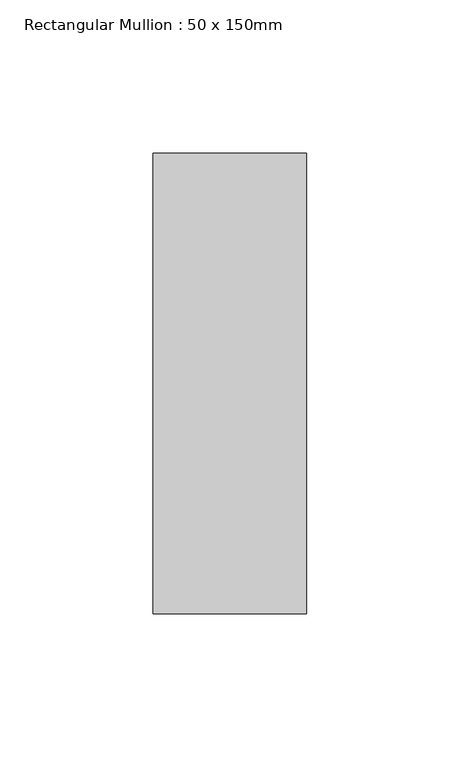
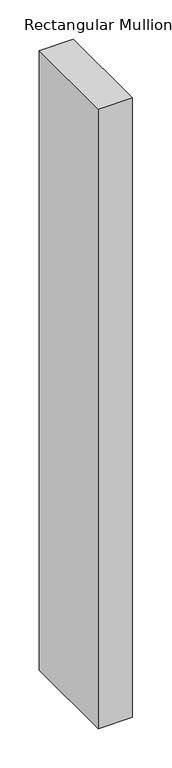
"""IFC4 building model written with IfcOpenShell, lengths in millimetres: member geometry, Rectangular Mullion : 50 x 150mm."""

from ifc_helpers import new_model, si_unit, frame, origin, place, context, project, spatial, polyline, outline, extrude, source, transform, mapped, element, save


def rectangular_mullion_50_x_150mm_a74c1b10(model_context):
    return source(origin(), model_context, "Body", "SweptSolid", [
        extrude(outline(polyline([(0.0, 75.0), (0.0, -75.0), (-50.0, -75.0), (-50.0, 75.0), (0.0, 75.0)])), frame((0.0, 0.0, -962.5000002), z_axis=(0.0, 0.0, 1.0), x_axis=(1.0, 0.0, 0.0)), (0.0, 0.0, 1.0), 962.5000002),
    ])


if __name__ == "__main__":
    model = new_model("IFC4")
    model_context = context("Model", 3, world=origin())
    ifc_project = project(units=[si_unit("LENGTHUNIT", "METRE", prefix="MILLI")], contexts=[model_context])
    site = spatial("IfcSite", under=ifc_project)
    building = spatial("IfcBuilding", under=site)
    placement = place(None, origin())
    rectangular_mullion_50_x_150mm_shape = rectangular_mullion_50_x_150mm_a74c1b10(model_context)
    element("IfcMember", 1, ObjectType="Rectangular Mullion : 50 x 150mm", at=placement, inside=building, context=model_context, shape_type="MappedRepresentation", body=[
        mapped(rectangular_mullion_50_x_150mm_shape, transform((0.0, 0.0, 0.0), x_axis=(1.0, 0.0, 0.0), y_axis=(0.0, 1.0, 0.0), z_axis=(0.0, 0.0, 1.0))),
    ])
    save(model, "model.ifc")

# Revit data of these elements
# Type "Rectangular Mullion : 50 x 150mm"
#   built-in parameter 1007304 = 0.492126 (stored number, unit not read)
#   built-in parameter 1007301 = 0.082021 (stored number, unit not read)
#   built-in parameter 1007300 = 0.082021 (stored number, unit not read)
# Element 1 (IfcMember, "Rectangular Mullion : 50 x 150mm")
#   Materials on its faces: "Aluminium"
# Materials
#   "Aluminium": class "Metal", colour RGB 247 247 247, transparency 0, Description = "Aluminium 6061", Cost = 0
